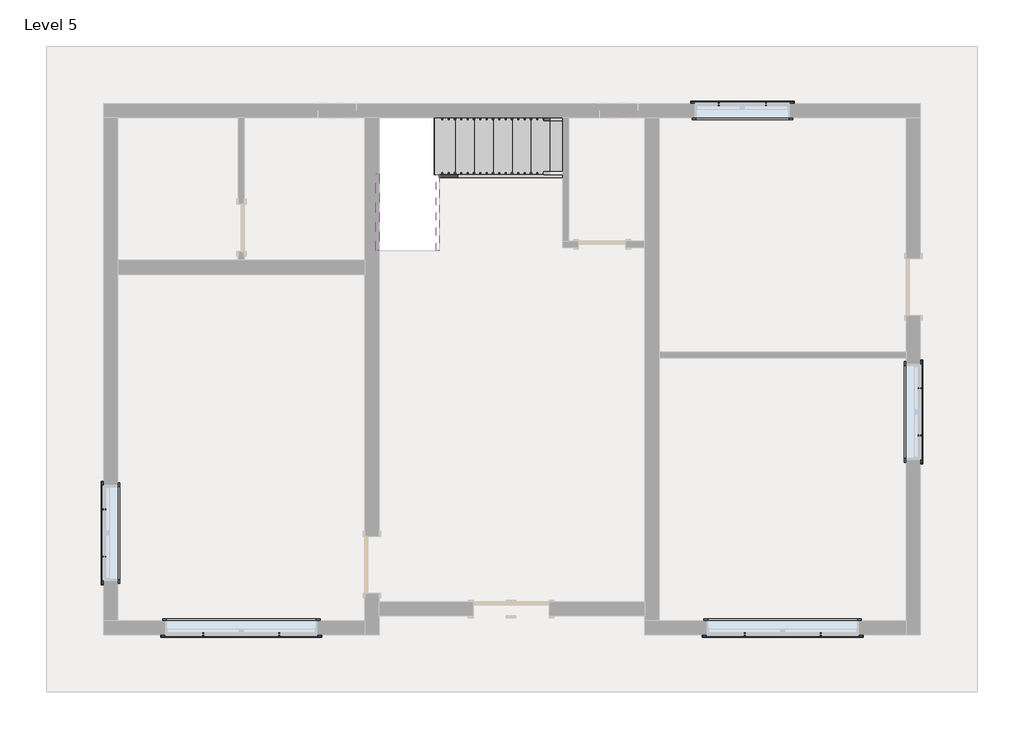
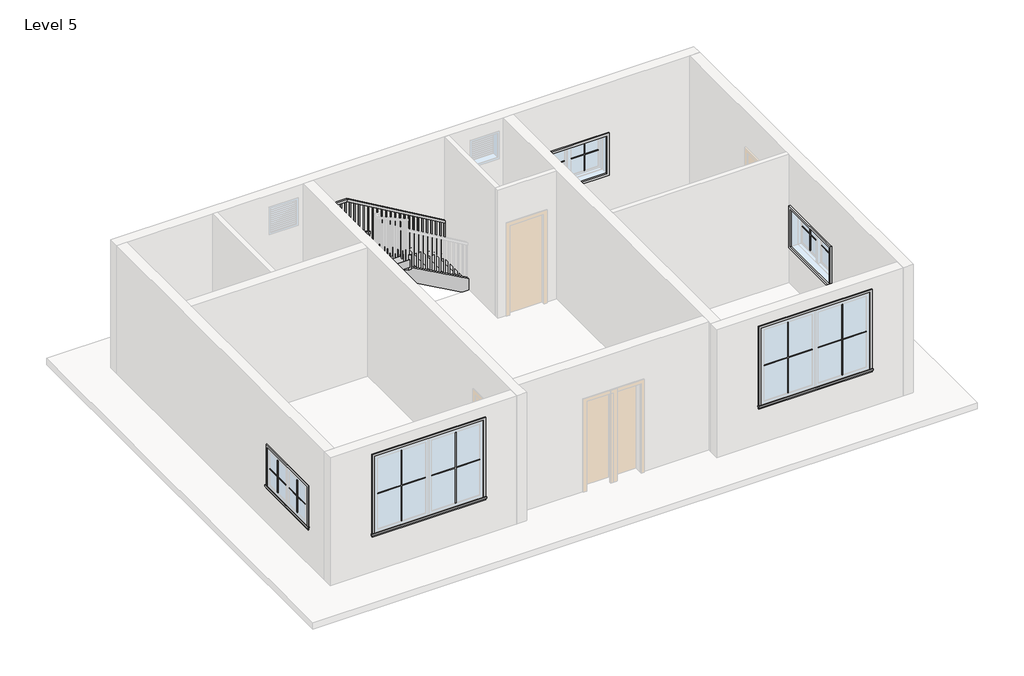
# One storey, part 2 of 2: 20 proxies, 4 members, 1 railing, 1 stair flight.
"""IFC4 building model written with IfcOpenShell, lengths in millimetres."""

from ifc_helpers import new_model, si_unit, frame, origin, place, context, project, spatial, polyline, outline, extrude, faceted_brep, transform, mapped, element, save
from components import muntin_pattern_2x2_muntin_pattern_2x2_9352d081, muntin_pattern_2x2_muntin_pattern_2x2_5c2cbe28, muntin_pattern_2x2_muntin_pattern_2x2_bb8d4d84, muntin_pattern_2x2_muntin_pattern_2x2_d03a1f3c, trim_window_exterior_flat_with_sill_979bde60, trim_window_exterior_flat_with_sill_359ed2ce, trim_window_interior_flat_picture_frame_7883d11b, trim_window_interior_flat_picture_frame_939a8053, stair_flight_cb1a632b

model = new_model("IFC4")

# Units and contexts
model_context = context("Model", 3, world=origin())
ifc_project = project(units=[si_unit("LENGTHUNIT", "METRE", prefix="MILLI")], contexts=[model_context])

# Site, building, storey
site = spatial("IfcSite", under=ifc_project)
building = spatial("IfcBuilding", under=site)
storey = spatial("IfcBuildingStorey", under=building, Name="Level 5", Elevation=12649.2)

# Proxies
placement = place(None, origin())
muntin_pattern_2x2_muntin_pattern_2x2_shape = muntin_pattern_2x2_muntin_pattern_2x2_9352d081(model_context)
element("IfcBuildingElementProxy", 1, Name="Muntin Pattern_2x2 : Muntin Pattern_2x2", ObjectType="Muntin Pattern_2x2 : Muntin Pattern_2x2", at=placement, inside=storey, context=model_context, shape_type="MappedRepresentation", body=[
    mapped(muntin_pattern_2x2_muntin_pattern_2x2_shape, transform((-7798.9165084, -1764.5743005, 13633.45), x_axis=(0.0, 1.0, 0.0), y_axis=(-1.0, 0.0, 0.0), z_axis=(0.0, 0.0, 1.0))),
])
element("IfcBuildingElementProxy", 2, Name="Muntin Pattern_2x2 : Muntin Pattern_2x2", ObjectType="Muntin Pattern_2x2 : Muntin Pattern_2x2", at=placement, inside=storey, context=model_context, shape_type="MappedRepresentation", body=[
    mapped(muntin_pattern_2x2_muntin_pattern_2x2_shape, transform((5288.4334916, 937.3506995, 13633.45), x_axis=(0.0, -1.0, 0.0), y_axis=(1.0, 0.0, 0.0), z_axis=(0.0, 0.0, 1.0))),
])
element("IfcBuildingElementProxy", 3, Name="Muntin Pattern_2x2 : Muntin Pattern_2x2", ObjectType="Muntin Pattern_2x2 : Muntin Pattern_2x2", at=placement, inside=storey, context=model_context, shape_type="MappedRepresentation", body=[
    mapped(muntin_pattern_2x2_muntin_pattern_2x2_shape, transform((2061.0459916, 5501.4131995, 13633.45), x_axis=(1.0, 0.0, 0.0), y_axis=(0.0, 1.0, 0.0), z_axis=(0.0, 0.0, 1.0))),
])
muntin_pattern_2x2_muntin_pattern_2x2_2_shape = muntin_pattern_2x2_muntin_pattern_2x2_5c2cbe28(model_context)
element("IfcBuildingElementProxy", 4, Name="Muntin Pattern_2x2 : Muntin Pattern_2x2", ObjectType="Muntin Pattern_2x2 : Muntin Pattern_2x2", at=placement, inside=storey, context=model_context, shape_type="MappedRepresentation", body=[
    mapped(muntin_pattern_2x2_muntin_pattern_2x2_2_shape, transform((-7798.9165084, -1005.7493005, 13633.45), x_axis=(0.0, -1.0, 0.0), y_axis=(1.0, 0.0, 0.0), z_axis=(0.0, 0.0, 1.0))),
])
element("IfcBuildingElementProxy", 5, Name="Muntin Pattern_2x2 : Muntin Pattern_2x2", ObjectType="Muntin Pattern_2x2 : Muntin Pattern_2x2", at=placement, inside=storey, context=model_context, shape_type="MappedRepresentation", body=[
    mapped(muntin_pattern_2x2_muntin_pattern_2x2_2_shape, transform((5288.4334916, 178.5256995, 13633.45), x_axis=(0.0, 1.0, 0.0), y_axis=(-1.0, 0.0, 0.0), z_axis=(0.0, 0.0, 1.0))),
])
element("IfcBuildingElementProxy", 6, Name="Muntin Pattern_2x2 : Muntin Pattern_2x2", ObjectType="Muntin Pattern_2x2 : Muntin Pattern_2x2", at=placement, inside=storey, context=model_context, shape_type="MappedRepresentation", body=[
    mapped(muntin_pattern_2x2_muntin_pattern_2x2_2_shape, transform((2819.8709916, 5501.4131995, 13633.45), x_axis=(-1.0, 0.0, 0.0), y_axis=(0.0, -1.0, 0.0), z_axis=(0.0, 0.0, 1.0))),
])
muntin_pattern_2x2_muntin_pattern_2x2_3_shape = muntin_pattern_2x2_muntin_pattern_2x2_bb8d4d84(model_context)
element("IfcBuildingElementProxy", 7, Name="Muntin Pattern_2x2 : Muntin Pattern_2x2", ObjectType="Muntin Pattern_2x2 : Muntin Pattern_2x2", at=placement, inside=storey, context=model_context, shape_type="MappedRepresentation", body=[
    mapped(muntin_pattern_2x2_muntin_pattern_2x2_3_shape, transform((-4990.6290084, -3013.9368005, 13633.45), x_axis=(-1.0, 0.0, 0.0), y_axis=(0.0, -1.0, 0.0), z_axis=(0.0, 0.0, 1.0))),
])
element("IfcBuildingElementProxy", 8, Name="Muntin Pattern_2x2 : Muntin Pattern_2x2", ObjectType="Muntin Pattern_2x2 : Muntin Pattern_2x2", at=placement, inside=storey, context=model_context, shape_type="MappedRepresentation", body=[
    mapped(muntin_pattern_2x2_muntin_pattern_2x2_3_shape, transform((3696.1709916, -3013.9368005, 13633.45), x_axis=(-1.0, 0.0, 0.0), y_axis=(0.0, -1.0, 0.0), z_axis=(0.0, 0.0, 1.0))),
])
muntin_pattern_2x2_muntin_pattern_2x2_4_shape = muntin_pattern_2x2_muntin_pattern_2x2_d03a1f3c(model_context)
element("IfcBuildingElementProxy", 9, Name="Muntin Pattern_2x2 : Muntin Pattern_2x2", ObjectType="Muntin Pattern_2x2 : Muntin Pattern_2x2", at=placement, inside=storey, context=model_context, shape_type="MappedRepresentation", body=[
    mapped(muntin_pattern_2x2_muntin_pattern_2x2_4_shape, transform((-6206.6540084, -3013.9368005, 13633.45), x_axis=(1.0, 0.0, 0.0), y_axis=(0.0, 1.0, 0.0), z_axis=(0.0, 0.0, 1.0))),
])
element("IfcBuildingElementProxy", 10, Name="Muntin Pattern_2x2 : Muntin Pattern_2x2", ObjectType="Muntin Pattern_2x2 : Muntin Pattern_2x2", at=placement, inside=storey, context=model_context, shape_type="MappedRepresentation", body=[
    mapped(muntin_pattern_2x2_muntin_pattern_2x2_4_shape, transform((2480.1459916, -3013.9368005, 13633.45), x_axis=(1.0, 0.0, 0.0), y_axis=(0.0, 1.0, 0.0), z_axis=(0.0, 0.0, 1.0))),
])
trim_window_exterior_flat_with_sill_shape = trim_window_exterior_flat_with_sill_979bde60(model_context)
element("IfcBuildingElementProxy", 11, Name="Trim-Window-Exterior-Flat : with Sill", ObjectType="Trim-Window-Exterior-Flat : with Sill", at=placement, inside=storey, context=model_context, shape_type="MappedRepresentation", body=[
    mapped(trim_window_exterior_flat_with_sill_shape, transform((-7808.4415084, -1385.1618005, 14478.0), x_axis=(0.0, -1.0, 0.0), y_axis=(0.0, 0.0, 1.0), z_axis=(-1.0, 0.0, 0.0))),
])
element("IfcBuildingElementProxy", 12, Name="Trim-Window-Exterior-Flat : with Sill", ObjectType="Trim-Window-Exterior-Flat : with Sill", at=placement, inside=storey, context=model_context, shape_type="MappedRepresentation", body=[
    mapped(trim_window_exterior_flat_with_sill_shape, transform((5297.9584916, 557.9381995, 14478.0), x_axis=(0.0, 1.0, 0.0), y_axis=(0.0, 0.0, 1.0), z_axis=(1.0, 0.0, 0.0))),
])
element("IfcBuildingElementProxy", 13, Name="Trim-Window-Exterior-Flat : with Sill", ObjectType="Trim-Window-Exterior-Flat : with Sill", at=placement, inside=storey, context=model_context, shape_type="MappedRepresentation", body=[
    mapped(trim_window_exterior_flat_with_sill_shape, transform((2440.4584916, 5510.9381995, 14478.0), x_axis=(-1.0, 0.0, 0.0), y_axis=(0.0, 0.0, 1.0), z_axis=(0.0, 1.0, 0.0))),
])
trim_window_exterior_flat_with_sill_2_shape = trim_window_exterior_flat_with_sill_359ed2ce(model_context)
element("IfcBuildingElementProxy", 14, Name="Trim-Window-Exterior-Flat : with Sill", ObjectType="Trim-Window-Exterior-Flat : with Sill", at=placement, inside=storey, context=model_context, shape_type="MappedRepresentation", body=[
    mapped(trim_window_exterior_flat_with_sill_2_shape, transform((-5598.6415084, -3023.4618005, 15392.4), x_axis=(1.0, 0.0, 0.0), y_axis=(0.0, 0.0, 1.0), z_axis=(0.0, -1.0, 0.0))),
])
element("IfcBuildingElementProxy", 15, Name="Trim-Window-Exterior-Flat : with Sill", ObjectType="Trim-Window-Exterior-Flat : with Sill", at=placement, inside=storey, context=model_context, shape_type="MappedRepresentation", body=[
    mapped(trim_window_exterior_flat_with_sill_2_shape, transform((3088.1584916, -3023.4618005, 15392.4), x_axis=(1.0, 0.0, 0.0), y_axis=(0.0, 0.0, 1.0), z_axis=(0.0, -1.0, 0.0))),
])
trim_window_interior_flat_picture_frame_shape = trim_window_interior_flat_picture_frame_7883d11b(model_context)
element("IfcBuildingElementProxy", 16, Name="Trim-Window-Interior-Flat : Picture Frame", ObjectType="Trim-Window-Interior-Flat : Picture Frame", at=placement, inside=storey, context=model_context, shape_type="MappedRepresentation", body=[
    mapped(trim_window_interior_flat_picture_frame_shape, transform((-7579.8415084, -1385.1618005, 14478.0), x_axis=(0.0, 1.0, 0.0), y_axis=(0.0, 0.0, 1.0), z_axis=(1.0, 0.0, 0.0))),
])
element("IfcBuildingElementProxy", 17, Name="Trim-Window-Interior-Flat : Picture Frame", ObjectType="Trim-Window-Interior-Flat : Picture Frame", at=placement, inside=storey, context=model_context, shape_type="MappedRepresentation", body=[
    mapped(trim_window_interior_flat_picture_frame_shape, transform((5069.3584916, 557.9381995, 14478.0), x_axis=(0.0, -1.0, 0.0), y_axis=(0.0, 0.0, 1.0), z_axis=(-1.0, 0.0, 0.0))),
])
element("IfcBuildingElementProxy", 18, Name="Trim-Window-Interior-Flat : Picture Frame", ObjectType="Trim-Window-Interior-Flat : Picture Frame", at=placement, inside=storey, context=model_context, shape_type="MappedRepresentation", body=[
    mapped(trim_window_interior_flat_picture_frame_shape, transform((2440.4584916, 5282.3381995, 14478.0), x_axis=(1.0, 0.0, 0.0), y_axis=(0.0, 0.0, 1.0), z_axis=(0.0, -1.0, 0.0))),
])
trim_window_interior_flat_picture_frame_2_shape = trim_window_interior_flat_picture_frame_939a8053(model_context)
element("IfcBuildingElementProxy", 19, Name="Trim-Window-Interior-Flat : Picture Frame", ObjectType="Trim-Window-Interior-Flat : Picture Frame", at=placement, inside=storey, context=model_context, shape_type="MappedRepresentation", body=[
    mapped(trim_window_interior_flat_picture_frame_2_shape, transform((-5598.6415084, -2794.8618005, 15392.4), x_axis=(-1.0, 0.0, 0.0), y_axis=(0.0, 0.0, 1.0), z_axis=(0.0, 1.0, 0.0))),
])
element("IfcBuildingElementProxy", 20, Name="Trim-Window-Interior-Flat : Picture Frame", ObjectType="Trim-Window-Interior-Flat : Picture Frame", at=placement, inside=storey, context=model_context, shape_type="MappedRepresentation", body=[
    mapped(trim_window_interior_flat_picture_frame_2_shape, transform((3088.1584916, -2794.8618005, 15392.4), x_axis=(-1.0, 0.0, 0.0), y_axis=(0.0, 0.0, 1.0), z_axis=(0.0, 1.0, 0.0))),
])

# Members
element("IfcMember", 21, ObjectType="Stringer - 2\" Width", at=placement, inside=storey, context=model_context, shape_type="SweptSolid", body=[
    extrude(outline(polyline([(12649.2, -442.4415084), (12913.2428392, -442.4415084), (14013.9095059, -2423.6415084), (13665.2308318, -2423.6415084), (12649.2, -594.7860112), (12649.2, -442.4415084)])), frame((0.0, 4317.5146777, 0.0), z_axis=(0.0, 1.0, 0.0), x_axis=(0.0, 0.0, 1.0)), (0.0, 0.0, 1.0), 50.8),
])
element("IfcMember", 22, ObjectType="Stringer - 2\" Width", at=placement, inside=storey, context=model_context, shape_type="SweptSolid", body=[
    extrude(outline(polyline([(4368.3146777, 14211.445537), (4368.3146777, 13862.8006925), (3148.7383287, 14540.0643411), (3148.7383287, 14888.7091856), (4368.3146777, 14211.445537)])), frame((-2474.4415084, 0.0, 0.0), z_axis=(1.0, 0.0, 0.0), x_axis=(0.0, 1.0, 0.0)), (0.0, 0.0, 1.0), 50.8),
])
element("IfcMember", 23, ObjectType="Stringer - 2\" Width", at=placement, inside=storey, context=model_context, shape_type="SweptSolid", body=[
    extrude(outline(polyline([(12649.2, -442.4415084), (12913.2428392, -442.4415084), (13703.8636166, -1865.5589077), (13703.8636166, -2493.1805211), (12649.2, -594.7860112), (12649.2, -442.4415084)])), frame((0.0, 5282.3381995, 0.0), z_axis=(0.0, 1.0, 0.0), x_axis=(0.0, 0.0, 1.0)), (0.0, 0.0, 1.0), 50.8),
])
element("IfcMember", 24, ObjectType="Stringer - 2\" Width", at=placement, inside=storey, context=model_context, shape_type="SweptSolid", body=[
    extrude(outline(polyline([(3758.489521, 14201.453054), (3148.7383287, 14540.0643411), (3148.7383287, 14888.7091856), (4386.3085505, 14201.453054), (3758.489521, 14201.453054)])), frame((-3439.6415084, 0.0, 0.0), z_axis=(1.0, 0.0, 0.0), x_axis=(0.0, 1.0, 0.0)), (0.0, 0.0, 1.0), 50.8),
])

# Railing
element("IfcRailing", 25, ObjectType="Handrail - Rectangular", at=placement, inside=storey, context=model_context, shape_type="SolidModel", body=[
    faceted_brep([(-442.4415084, 5231.5381995, 13732.9333333), (-442.4415084, 5231.5381995, 13674.1219871), (-442.4415084, 5282.3381995, 13674.1219871), (-442.4415084, 5282.3381995, 13732.9333333), (-2641.0608886, 5231.5381995, 15015.4613051), (-2654.794625, 5231.5381995, 14964.6613051), (-2654.794625, 5282.3381995, 14964.6613051), (-2641.0608886, 5282.3381995, 15015.4613051), (-3338.0415084, 5231.5381995, 15015.4613051), (-3338.0415084, 5231.5381995, 14964.6613051), (-3388.8415084, 5282.3381995, 14964.6613051), (-3388.8415084, 5282.3381995, 15015.4613051), (-3338.0415084, 4498.2044111, 15015.4613051), (-3338.0415084, 4485.04436, 14964.6613051), (-3388.8415084, 4485.04436, 14964.6613051), (-3388.8415084, 4498.2044111, 15015.4613051), (-3338.0415084, 3148.7383287, 15764.9333333), (-3388.8415084, 3148.7383287, 15764.9333333), (-3388.8415084, 3148.7383287, 15706.82445), (-3338.0415084, 3148.7383287, 15706.82445)], [[[0, 1, 2, 3]], [[1, 0, 4, 5]], [[2, 1, 5, 6]], [[3, 2, 6, 7]], [[0, 3, 7, 4]], [[5, 4, 8, 9]], [[6, 5, 9, 10]], [[7, 6, 10, 11]], [[4, 7, 11, 8]], [[9, 8, 12, 13]], [[10, 9, 13, 14]], [[11, 10, 14, 15]], [[8, 11, 15, 12]], [[16, 17, 18, 19]], [[13, 12, 16, 19]], [[14, 13, 19, 18]], [[15, 14, 18, 17]], [[12, 15, 17, 16]]]),
    extrude(outline(polyline([(3215.4131995, 15669.7942858), (3234.4631995, 15659.2142183), (3234.4631995, 14681.2), (3215.4131995, 14681.2), (3215.4131995, 15669.7942858)])), frame((-3372.9665084, 0.0, 0.0), z_axis=(1.0, 0.0, 0.0), x_axis=(0.0, 1.0, 0.0)), (0.0, 0.0, 1.0), 19.05),
    extrude(outline(polyline([(3317.0131995, 15613.5240232), (3336.0631995, 15602.9439558), (3336.0631995, 14681.2), (3317.0131995, 14681.2), (3317.0131995, 15613.5240232)])), frame((-3372.9665084, 0.0, 0.0), z_axis=(1.0, 0.0, 0.0), x_axis=(0.0, 1.0, 0.0)), (0.0, 0.0, 1.0), 19.05),
    extrude(outline(polyline([(3418.6131995, 15557.0969969), (3437.6631995, 15546.5169295), (3437.6631995, 14681.2), (3418.6131995, 14681.2), (3418.6131995, 15557.0969969)])), frame((-3372.9665084, 0.0, 0.0), z_axis=(1.0, 0.0, 0.0), x_axis=(0.0, 1.0, 0.0)), (0.0, 0.0, 1.0), 19.05),
    extrude(outline(polyline([(3520.2131995, 15500.6699707), (3539.2631995, 15490.0899033), (3539.2631995, 14511.8666667), (3520.2131995, 14511.8666667), (3520.2131995, 15500.6699707)])), frame((-3372.9665084, 0.0, 0.0), z_axis=(1.0, 0.0, 0.0), x_axis=(0.0, 1.0, 0.0)), (0.0, 0.0, 1.0), 19.05),
    extrude(outline(polyline([(3621.8131995, 15444.1906899), (3640.8631995, 15433.6106224), (3640.8631995, 14511.8666667), (3621.8131995, 14511.8666667), (3621.8131995, 15444.1906899)])), frame((-3372.9665084, 0.0, 0.0), z_axis=(1.0, 0.0, 0.0), x_axis=(0.0, 1.0, 0.0)), (0.0, 0.0, 1.0), 19.05),
    extrude(outline(polyline([(3723.4131995, 15387.7636636), (3742.4631995, 15377.1835962), (3742.4631995, 14511.8666667), (3723.4131995, 14511.8666667), (3723.4131995, 15387.7636636)])), frame((-3372.9665084, 0.0, 0.0), z_axis=(1.0, 0.0, 0.0), x_axis=(0.0, 1.0, 0.0)), (0.0, 0.0, 1.0), 19.05),
    extrude(outline(polyline([(3825.0131995, 15331.3366374), (3844.0631995, 15320.7565699), (3844.0631995, 14342.5333333), (3825.0131995, 14342.5333333), (3825.0131995, 15331.3366374)])), frame((-3372.9665084, 0.0, 0.0), z_axis=(1.0, 0.0, 0.0), x_axis=(0.0, 1.0, 0.0)), (0.0, 0.0, 1.0), 19.05),
    extrude(outline(polyline([(3926.6131995, 15274.8573565), (3945.6631995, 15264.2772891), (3945.6631995, 14342.5333333), (3926.6131995, 14342.5333333), (3926.6131995, 15274.8573565)])), frame((-3372.9665084, 0.0, 0.0), z_axis=(1.0, 0.0, 0.0), x_axis=(0.0, 1.0, 0.0)), (0.0, 0.0, 1.0), 19.05),
    extrude(outline(polyline([(4028.2131995, 15218.4303303), (4047.2631995, 15207.8502629), (4047.2631995, 14342.5333333), (4028.2131995, 14342.5333333), (4028.2131995, 15218.4303303)])), frame((-3372.9665084, 0.0, 0.0), z_axis=(1.0, 0.0, 0.0), x_axis=(0.0, 1.0, 0.0)), (0.0, 0.0, 1.0), 19.05),
    extrude(outline(polyline([(4129.8131995, 15162.003304), (4148.8631995, 15151.4232366), (4148.8631995, 14173.2), (4129.8131995, 14173.2), (4129.8131995, 15162.003304)])), frame((-3372.9665084, 0.0, 0.0), z_axis=(1.0, 0.0, 0.0), x_axis=(0.0, 1.0, 0.0)), (0.0, 0.0, 1.0), 19.05),
    extrude(outline(polyline([(4231.4131995, 15105.5240232), (4250.4631995, 15094.9439558), (4250.4631995, 14173.2), (4231.4131995, 14173.2), (4231.4131995, 15105.5240232)])), frame((-3372.9665084, 0.0, 0.0), z_axis=(1.0, 0.0, 0.0), x_axis=(0.0, 1.0, 0.0)), (0.0, 0.0, 1.0), 19.05),
    extrude(outline(polyline([(4333.0131995, 15049.0969969), (4352.0631995, 15038.5169295), (4352.0631995, 14173.2), (4333.0131995, 14173.2), (4333.0131995, 15049.0969969)])), frame((-3372.9665084, 0.0, 0.0), z_axis=(1.0, 0.0, 0.0), x_axis=(0.0, 1.0, 0.0)), (0.0, 0.0, 1.0), 19.05),
    extrude(outline(polyline([(4434.6131995, 14992.6699707), (4453.6631995, 14982.0899033), (4453.6631995, 14003.8666667), (4434.6131995, 14003.8666667), (4434.6131995, 14992.6699707)])), frame((-3372.9665084, 0.0, 0.0), z_axis=(1.0, 0.0, 0.0), x_axis=(0.0, 1.0, 0.0)), (0.0, 0.0, 1.0), 19.05),
    extrude(outline(polyline([(-3372.9665084, 4555.2631995), (-3353.9165084, 4555.2631995), (-3353.9165084, 4536.2131995), (-3372.9665084, 4536.2131995), (-3372.9665084, 4555.2631995)])), frame((0.0, 0.0, 14003.8666667), z_axis=(0.0, 0.0, 1.0), x_axis=(1.0, 0.0, 0.0)), (0.0, 0.0, 1.0), 960.7946385),
    extrude(outline(polyline([(-3372.9665084, 4656.8631995), (-3353.9165084, 4656.8631995), (-3353.9165084, 4637.8131995), (-3372.9665084, 4637.8131995), (-3372.9665084, 4656.8631995)])), frame((0.0, 0.0, 14003.8666667), z_axis=(0.0, 0.0, 1.0), x_axis=(1.0, 0.0, 0.0)), (0.0, 0.0, 1.0), 960.7946385),
    extrude(outline(polyline([(-3372.9665084, 4758.4631995), (-3353.9165084, 4758.4631995), (-3353.9165084, 4739.4131995), (-3372.9665084, 4739.4131995), (-3372.9665084, 4758.4631995)])), frame((0.0, 0.0, 14003.8666667), z_axis=(0.0, 0.0, 1.0), x_axis=(1.0, 0.0, 0.0)), (0.0, 0.0, 1.0), 960.7946385),
    extrude(outline(polyline([(-3372.9665084, 4860.0631995), (-3353.9165084, 4860.0631995), (-3353.9165084, 4841.0131995), (-3372.9665084, 4841.0131995), (-3372.9665084, 4860.0631995)])), frame((0.0, 0.0, 14003.8666667), z_axis=(0.0, 0.0, 1.0), x_axis=(1.0, 0.0, 0.0)), (0.0, 0.0, 1.0), 960.7946385),
    extrude(outline(polyline([(-3372.9665084, 4961.6631995), (-3353.9165084, 4961.6631995), (-3353.9165084, 4942.6131995), (-3372.9665084, 4942.6131995), (-3372.9665084, 4961.6631995)])), frame((0.0, 0.0, 14003.8666667), z_axis=(0.0, 0.0, 1.0), x_axis=(1.0, 0.0, 0.0)), (0.0, 0.0, 1.0), 960.7946385),
    extrude(outline(polyline([(-3372.9665084, 5063.2631995), (-3353.9165084, 5063.2631995), (-3353.9165084, 5044.2131995), (-3372.9665084, 5044.2131995), (-3372.9665084, 5063.2631995)])), frame((0.0, 0.0, 14003.8666667), z_axis=(0.0, 0.0, 1.0), x_axis=(1.0, 0.0, 0.0)), (0.0, 0.0, 1.0), 960.7946385),
    extrude(outline(polyline([(-3372.9665084, 5164.8631995), (-3353.9165084, 5164.8631995), (-3353.9165084, 5145.8131995), (-3372.9665084, 5145.8131995), (-3372.9665084, 5164.8631995)])), frame((0.0, 0.0, 14003.8666667), z_axis=(0.0, 0.0, 1.0), x_axis=(1.0, 0.0, 0.0)), (0.0, 0.0, 1.0), 960.7946385),
    extrude(outline(polyline([(-3277.7165084, 5266.4631995), (-3277.7165084, 5247.4131995), (-3296.7665084, 5247.4131995), (-3296.7665084, 5266.4631995), (-3277.7165084, 5266.4631995)])), frame((0.0, 0.0, 14003.8666667), z_axis=(0.0, 0.0, 1.0), x_axis=(1.0, 0.0, 0.0)), (0.0, 0.0, 1.0), 960.7946385),
    extrude(outline(polyline([(-3176.1165084, 5266.4631995), (-3176.1165084, 5247.4131995), (-3195.1665084, 5247.4131995), (-3195.1665084, 5266.4631995), (-3176.1165084, 5266.4631995)])), frame((0.0, 0.0, 14003.8666667), z_axis=(0.0, 0.0, 1.0), x_axis=(1.0, 0.0, 0.0)), (0.0, 0.0, 1.0), 960.7946385),
    extrude(outline(polyline([(-3074.5165084, 5266.4631995), (-3074.5165084, 5247.4131995), (-3093.5665084, 5247.4131995), (-3093.5665084, 5266.4631995), (-3074.5165084, 5266.4631995)])), frame((0.0, 0.0, 14003.8666667), z_axis=(0.0, 0.0, 1.0), x_axis=(1.0, 0.0, 0.0)), (0.0, 0.0, 1.0), 960.7946385),
    extrude(outline(polyline([(-2972.9165084, 5266.4631995), (-2972.9165084, 5247.4131995), (-2991.9665084, 5247.4131995), (-2991.9665084, 5266.4631995), (-2972.9165084, 5266.4631995)])), frame((0.0, 0.0, 14003.8666667), z_axis=(0.0, 0.0, 1.0), x_axis=(1.0, 0.0, 0.0)), (0.0, 0.0, 1.0), 960.7946385),
    extrude(outline(polyline([(-2871.3165084, 5266.4631995), (-2871.3165084, 5247.4131995), (-2890.3665084, 5247.4131995), (-2890.3665084, 5266.4631995), (-2871.3165084, 5266.4631995)])), frame((0.0, 0.0, 14003.8666667), z_axis=(0.0, 0.0, 1.0), x_axis=(1.0, 0.0, 0.0)), (0.0, 0.0, 1.0), 960.7946385),
    extrude(outline(polyline([(-2769.7165084, 5266.4631995), (-2769.7165084, 5247.4131995), (-2788.7665084, 5247.4131995), (-2788.7665084, 5266.4631995), (-2769.7165084, 5266.4631995)])), frame((0.0, 0.0, 14003.8666667), z_axis=(0.0, 0.0, 1.0), x_axis=(1.0, 0.0, 0.0)), (0.0, 0.0, 1.0), 960.7946385),
    extrude(outline(polyline([(-2668.1165084, 5266.4631995), (-2668.1165084, 5247.4131995), (-2687.1665084, 5247.4131995), (-2687.1665084, 5266.4631995), (-2668.1165084, 5266.4631995)])), frame((0.0, 0.0, 14003.8666667), z_axis=(0.0, 0.0, 1.0), x_axis=(1.0, 0.0, 0.0)), (0.0, 0.0, 1.0), 960.7946385),
    extrude(outline(polyline([(14913.1657371, -2566.5165084), (14924.2782371, -2585.5665084), (14003.8666667, -2585.5665084), (14003.8666667, -2566.5165084), (14913.1657371, -2566.5165084)])), frame((0.0, 5247.4131995, 0.0), z_axis=(0.0, 1.0, 0.0), x_axis=(0.0, 0.0, 1.0)), (0.0, 0.0, 1.0), 19.05),
    extrude(outline(polyline([(14853.8990704, -2464.9165084), (14865.0115704, -2483.9665084), (14003.8666667, -2483.9665084), (14003.8666667, -2464.9165084), (14853.8990704, -2464.9165084)])), frame((0.0, 5247.4131995, 0.0), z_axis=(0.0, 1.0, 0.0), x_axis=(0.0, 0.0, 1.0)), (0.0, 0.0, 1.0), 19.05),
    extrude(outline(polyline([(14794.6324038, -2363.3165084), (14805.7449038, -2382.3665084), (13834.5333333, -2382.3665084), (13834.5333333, -2363.3165084), (14794.6324038, -2363.3165084)])), frame((0.0, 5247.4131995, 0.0), z_axis=(0.0, 1.0, 0.0), x_axis=(0.0, 0.0, 1.0)), (0.0, 0.0, 1.0), 19.05),
    extrude(outline(polyline([(14735.3657371, -2261.7165084), (14746.4782371, -2280.7665084), (13834.5333333, -2280.7665084), (13834.5333333, -2261.7165084), (14735.3657371, -2261.7165084)])), frame((0.0, 5247.4131995, 0.0), z_axis=(0.0, 1.0, 0.0), x_axis=(0.0, 0.0, 1.0)), (0.0, 0.0, 1.0), 19.05),
    extrude(outline(polyline([(14676.0990704, -2160.1165084), (14687.2115704, -2179.1665084), (13834.5333333, -2179.1665084), (13834.5333333, -2160.1165084), (14676.0990704, -2160.1165084)])), frame((0.0, 5247.4131995, 0.0), z_axis=(0.0, 1.0, 0.0), x_axis=(0.0, 0.0, 1.0)), (0.0, 0.0, 1.0), 19.05),
    extrude(outline(polyline([(14616.8324038, -2058.5165084), (14627.9449038, -2077.5665084), (13665.2, -2077.5665084), (13665.2, -2058.5165084), (14616.8324038, -2058.5165084)])), frame((0.0, 5247.4131995, 0.0), z_axis=(0.0, 1.0, 0.0), x_axis=(0.0, 0.0, 1.0)), (0.0, 0.0, 1.0), 19.05),
    extrude(outline(polyline([(14557.5657371, -1956.9165084), (14568.6782371, -1975.9665084), (13665.2, -1975.9665084), (13665.2, -1956.9165084), (14557.5657371, -1956.9165084)])), frame((0.0, 5247.4131995, 0.0), z_axis=(0.0, 1.0, 0.0), x_axis=(0.0, 0.0, 1.0)), (0.0, 0.0, 1.0), 19.05),
    extrude(outline(polyline([(14498.2990704, -1855.3165084), (14509.4115704, -1874.3665084), (13665.2, -1874.3665084), (13665.2, -1855.3165084), (14498.2990704, -1855.3165084)])), frame((0.0, 5247.4131995, 0.0), z_axis=(0.0, 1.0, 0.0), x_axis=(0.0, 0.0, 1.0)), (0.0, 0.0, 1.0), 19.05),
    extrude(outline(polyline([(14439.0324038, -1753.7165084), (14450.1449038, -1772.7665084), (13495.8666667, -1772.7665084), (13495.8666667, -1753.7165084), (14439.0324038, -1753.7165084)])), frame((0.0, 5247.4131995, 0.0), z_axis=(0.0, 1.0, 0.0), x_axis=(0.0, 0.0, 1.0)), (0.0, 0.0, 1.0), 19.05),
    extrude(outline(polyline([(14379.7657371, -1652.1165084), (14390.8782371, -1671.1665084), (13495.8666667, -1671.1665084), (13495.8666667, -1652.1165084), (14379.7657371, -1652.1165084)])), frame((0.0, 5247.4131995, 0.0), z_axis=(0.0, 1.0, 0.0), x_axis=(0.0, 0.0, 1.0)), (0.0, 0.0, 1.0), 19.05),
    extrude(outline(polyline([(14320.4990704, -1550.5165084), (14331.6115704, -1569.5665084), (13495.8666667, -1569.5665084), (13495.8666667, -1550.5165084), (14320.4990704, -1550.5165084)])), frame((0.0, 5247.4131995, 0.0), z_axis=(0.0, 1.0, 0.0), x_axis=(0.0, 0.0, 1.0)), (0.0, 0.0, 1.0), 19.05),
    extrude(outline(polyline([(14261.2324038, -1448.9165084), (14272.3449038, -1467.9665084), (13326.5333333, -1467.9665084), (13326.5333333, -1448.9165084), (14261.2324038, -1448.9165084)])), frame((0.0, 5247.4131995, 0.0), z_axis=(0.0, 1.0, 0.0), x_axis=(0.0, 0.0, 1.0)), (0.0, 0.0, 1.0), 19.05),
    extrude(outline(polyline([(14201.9657371, -1347.3165084), (14213.0782371, -1366.3665084), (13326.5333333, -1366.3665084), (13326.5333333, -1347.3165084), (14201.9657371, -1347.3165084)])), frame((0.0, 5247.4131995, 0.0), z_axis=(0.0, 1.0, 0.0), x_axis=(0.0, 0.0, 1.0)), (0.0, 0.0, 1.0), 19.05),
    extrude(outline(polyline([(14142.6990704, -1245.7165084), (14153.8115704, -1264.7665084), (13326.5333333, -1264.7665084), (13326.5333333, -1245.7165084), (14142.6990704, -1245.7165084)])), frame((0.0, 5247.4131995, 0.0), z_axis=(0.0, 1.0, 0.0), x_axis=(0.0, 0.0, 1.0)), (0.0, 0.0, 1.0), 19.05),
    extrude(outline(polyline([(14083.4324038, -1144.1165084), (14094.5449038, -1163.1665084), (13157.2, -1163.1665084), (13157.2, -1144.1165084), (14083.4324038, -1144.1165084)])), frame((0.0, 5247.4131995, 0.0), z_axis=(0.0, 1.0, 0.0), x_axis=(0.0, 0.0, 1.0)), (0.0, 0.0, 1.0), 19.05),
    extrude(outline(polyline([(14024.1657371, -1042.5165084), (14035.2782371, -1061.5665084), (13157.2, -1061.5665084), (13157.2, -1042.5165084), (14024.1657371, -1042.5165084)])), frame((0.0, 5247.4131995, 0.0), z_axis=(0.0, 1.0, 0.0), x_axis=(0.0, 0.0, 1.0)), (0.0, 0.0, 1.0), 19.05),
    extrude(outline(polyline([(13964.8990704, -940.9165084), (13976.0115704, -959.9665084), (13157.2, -959.9665084), (13157.2, -940.9165084), (13964.8990704, -940.9165084)])), frame((0.0, 5247.4131995, 0.0), z_axis=(0.0, 1.0, 0.0), x_axis=(0.0, 0.0, 1.0)), (0.0, 0.0, 1.0), 19.05),
    extrude(outline(polyline([(13905.6324038, -839.3165084), (13916.7449038, -858.3665084), (12987.8666667, -858.3665084), (12987.8666667, -839.3165084), (13905.6324038, -839.3165084)])), frame((0.0, 5247.4131995, 0.0), z_axis=(0.0, 1.0, 0.0), x_axis=(0.0, 0.0, 1.0)), (0.0, 0.0, 1.0), 19.05),
    extrude(outline(polyline([(13846.3657371, -737.7165084), (13857.4782371, -756.7665084), (12987.8666667, -756.7665084), (12987.8666667, -737.7165084), (13846.3657371, -737.7165084)])), frame((0.0, 5247.4131995, 0.0), z_axis=(0.0, 1.0, 0.0), x_axis=(0.0, 0.0, 1.0)), (0.0, 0.0, 1.0), 19.05),
    extrude(outline(polyline([(13787.0990704, -636.1165084), (13798.2115704, -655.1665084), (12987.8666667, -655.1665084), (12987.8666667, -636.1165084), (13787.0990704, -636.1165084)])), frame((0.0, 5247.4131995, 0.0), z_axis=(0.0, 1.0, 0.0), x_axis=(0.0, 0.0, 1.0)), (0.0, 0.0, 1.0), 19.05),
    extrude(outline(polyline([(13727.8324038, -534.5165084), (13738.9449038, -553.5665084), (12818.5333333, -553.5665084), (12818.5333333, -534.5165084), (13727.8324038, -534.5165084)])), frame((0.0, 5247.4131995, 0.0), z_axis=(0.0, 1.0, 0.0), x_axis=(0.0, 0.0, 1.0)), (0.0, 0.0, 1.0), 19.05),
    extrude(outline(polyline([(-3353.9165084, 5266.4631995), (-3353.9165084, 5247.4131995), (-3372.9665084, 5247.4131995), (-3372.9665084, 5266.4631995), (-3353.9165084, 5266.4631995)])), frame((0.0, 0.0, 14003.8666667), z_axis=(0.0, 0.0, 1.0), x_axis=(1.0, 0.0, 0.0)), (0.0, 0.0, 1.0), 960.7946385),
    extrude(outline(polyline([(3148.7383287, 15706.82445), (3167.7883287, 15696.2443826), (3167.7883287, 14681.2), (3148.7383287, 14681.2), (3148.7383287, 15706.82445)])), frame((-3372.9665084, 0.0, 0.0), z_axis=(1.0, 0.0, 0.0), x_axis=(0.0, 1.0, 0.0)), (0.0, 0.0, 1.0), 19.05),
    extrude(outline(polyline([(13674.1219871, -442.4415084), (13685.2344871, -461.4915084), (12818.5333333, -461.4915084), (12818.5333333, -442.4415084), (13674.1219871, -442.4415084)])), frame((0.0, 5247.4131995, 0.0), z_axis=(0.0, 1.0, 0.0), x_axis=(0.0, 0.0, 1.0)), (0.0, 0.0, 1.0), 19.05),
])

# Stair flight
stair_flight_shape = stair_flight_cb1a632b(model_context)
element("IfcStairFlight", 26, ObjectType="2\" Tread 1\" Nosing 1/4\" Riser", at=placement, inside=storey, context=model_context, shape_type="MappedRepresentation", body=[
    mapped(stair_flight_shape, transform((0.0, 0.0, 0.0), x_axis=(1.0, 0.0, 0.0), y_axis=(0.0, 1.0, 0.0), z_axis=(0.0, 0.0, 1.0))),
])

save(model, "model.ifc")

# Revit data of these elements
# Type "Muntin Pattern_2x2 : Muntin Pattern_2x2"
#   Width [instance default] = 4' - 0"
#   Thickness = 0' - 0 1/2"
#   Height [instance default] = 4' - 0"
#   Distance = 0' - 0 3/4"
#   Interior Material [instance default] = none
#   Exterior Material [instance default] = none
#   Default Elevation = 0
# Type "Trim-Window-Exterior-Flat : with Sill"
#   Trim Width = 0' - 2 1/4"
#   Trim Thickness_Picture Frame = 0' - 1 1/4"
#   Trim Thickness_with Sill = 0' - 0 3/4"
#   Sill Thickness = 0' - 1 1/4"
#   Opening Width [instance default] = 2' - 0"
#   Opening Height [instance default] = 3' - 0"
#   Default Elevation = 4' - 0"
#   Sill = yes
#   Picture Frame = no
#   Trim Material [instance default] = none
# Type "Trim-Window-Interior-Flat : Picture Frame"
#   Trim Thickness_Picture Frame = 0' - 1 1/4"
#   Trim Width = 0' - 2 1/4"
#   Trim Thickness_with Sill = 0' - 0 3/4"
#   Sill Thickness = 0' - 1 1/4"
#   Opening Width [instance default] = 2' - 0"
#   Opening Height [instance default] = 3' - 0"
#   Default Elevation = 4' - 0"
#   Sill = no
#   Picture Frame = yes
#   Trim Material [instance default] = none
# Type "Handrail - Rectangular"
#   Assembly Code = "C2010400"
#   built-in parameter 1008612 = 0.0416667 (stored number, unit not read)
#   built-in parameter 1008611 = 0.0416667 (stored number, unit not read)
#   built-in parameter 1008609 = 0.333333 (stored number, unit not read)
#   built-in parameter 1008604 = 0.166667 (stored number, unit not read)
#   built-in parameter 1008603 = 0.166667 (stored number, unit not read)
#   Railing Height = 3' - 0"
#   built-in parameter 1008630 = 2
#   built-in parameter 1008610 = 2
#   built-in parameter 1008618 = Baluster - Square : 3/4"
# Elements 1, 2, 3, 4, 5, 6 (IfcBuildingElementProxy, "Muntin Pattern_2x2 : Muntin Pattern_2x2")
#   Width = 2' - 0 5/8"
#   Height = 2' - 6 1/2"
#   Interior Material = Wood - Stained
#   Exterior Material = Clad - White
#   Phase Created = New Construction
#   Materials on its faces: "Clad - White", "Wood - Stained"
# Elements 7, 8, 9, 10 (IfcBuildingElementProxy, "Muntin Pattern_2x2 : Muntin Pattern_2x2")
#   Width = 3' - 6 5/8"
#   Height = 5' - 6 1/2"
#   Interior Material = Wood - Stained
#   Exterior Material = Clad - White
#   Phase Created = New Construction
#   Materials on its faces: "Clad - White", "Wood - Stained"
# Elements 11, 12, 13 (IfcBuildingElementProxy, "Trim-Window-Exterior-Flat : with Sill")
#   Opening Width = 5' - 0"
#   Opening Height = 3' - 0"
#   Trim Material = Clad - White
#   Phase Created = New Construction
#   Materials on its faces: "Clad - White"
# Elements 14, 15 (IfcBuildingElementProxy, "Trim-Window-Exterior-Flat : with Sill")
#   Opening Width = 8' - 0"
#   Opening Height = 6' - 0"
#   Trim Material = Clad - White
#   Phase Created = New Construction
#   Materials on its faces: "Clad - White"
# Elements 16, 17, 18 (IfcBuildingElementProxy, "Trim-Window-Interior-Flat : Picture Frame")
#   Opening Width = 5' - 0"
#   Opening Height = 3' - 0"
#   Trim Material = Wood - Stained
#   Phase Created = New Construction
#   Materials on its faces: "Wood - Stained"
# Elements 19, 20 (IfcBuildingElementProxy, "Trim-Window-Interior-Flat : Picture Frame")
#   Opening Width = 8' - 0"
#   Opening Height = 6' - 0"
#   Trim Material = Wood - Stained
#   Phase Created = New Construction
#   Materials on its faces: "Wood - Stained"
# Elements 21, 22, 23, 24 (IfcMember, "Stringer - 2\" Width")
#   Phase Created = New Construction
# Element 25 (IfcRailing, "Handrail - Rectangular")
#   Phase Created = New Construction
# Element 26 (IfcStairFlight, "2\" Tread 1\" Nosing 1/4\" Riser")
#   Phase Created = New Construction
# Materials
#   "Clad - White": class "Wood", colour RGB 242 242 238, transparency 0, Cost = 0
#   "Wood - Stained": class "Wood", colour RGB 224 178 126, transparency 0, Cost = 0
